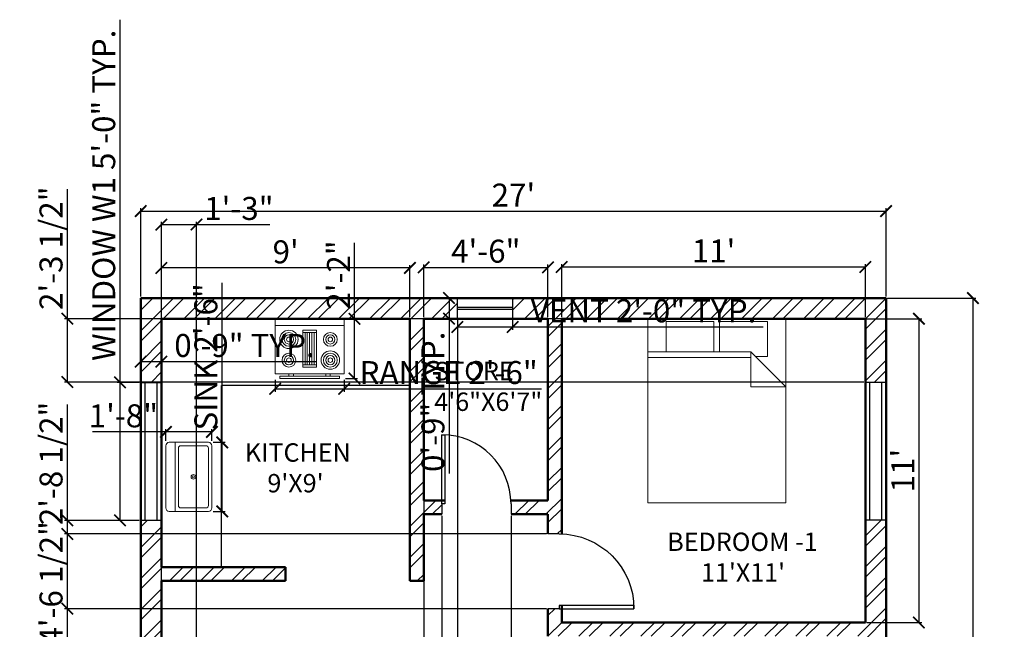
# Model space of a CAD drawing. Units: inches. Extents: x 9 to 670, y -4 to 628.
# Tile 2 of 2: x 9 to 437, y 363 to 628. Entities that reach past the tile are written whole.
import ezdxf

# ---------------------------------------------------------------- set-up
doc = ezdxf.new("R2010")
doc.units = ezdxf.units.IN
for name, color, linetype, lineweight in [('A-AREA-IDEN', 1, 'Continuous', 25), ('A-EQPM', 2, 'Continuous', 18), ('A-FLOR-CASE', 34, 'Continuous', 25), ('A-FLOR-FIXT', 2, 'Continuous', 18), ('A-FURN', 2, 'Continuous', 18), ('A-WALL-PATT', 9, 'Continuous', 13), ('DIM', 3, 'Continuous', 18), ('DOORS', 4, 'Continuous', 25), ('VENTILATOR', 11, 'Continuous', 25), ('WALLS', 6, 'Continuous', 50), ('WINDOWS', 20, 'Continuous', 25)]:
    doc.layers.add(name, color=color, linetype=linetype, lineweight=lineweight)
doc.styles.get("Standard").update_dxf_attribs({"font": 'arial.ttf'})
doc.dimstyles.new('ISO-25', dxfattribs={"dimtxt": 10, "dimasz": 5, "dimexe": 1.25, "dimexo": 0.625, "dimtad": 1, "dimlunit": 4, "dimtxsty": 'Standard', "dimblk": 'ARCHTICK', "dimcen": 2.5, "dimadec": 0, "dimazin": 0, "dimtfac": 1, "dimtmove": 0, "dimatfit": 3, "dimfxl": 1, "dimarcsym": 0})

# ---------------------------------------------------------------- blocks, each defined once
blk = doc.blocks.new('Bed - Queen')
for p, q in [((0, -80.00003), (0, 0)), ((0, 0), (59.99999, 0)), ((59.99999, 0), (59.99999, -80.00003)), ((7.99999, -1.2), (28.79998, -1.2)), ((7.99999, -14.4), (7.99999, -1.2)), ((28.79998, -1.2), (28.79998, -14.4)), ((31.19999, -1.2), (51.99999, -1.2)), ((31.19999, -14.4), (31.19999, -1.2)), ((51.99999, -1.2), (51.99999, -16.4)), ((0, -14.4), (44.8, -14.4)), ((44.8, -16.8), (0, -16.8)), ((59.99999, -29.6), (44.8, -14.4)), ((44.8, -14.4), (44.8, -29.6)), ((51.99999, -16.4), (46.79936, -16.4)), ((44.8, -29.6), (59.99999, -29.6)), ((59.99999, -80.00003), (0, -80.00003))]:
    blk.add_line(p, q)
blk = doc.blocks.new('Sink-single - 30 in top')
blk.add_line((-15, -3.999996), (15, -3.999996))
for points in [[(-13.5, 0), (13.5, 0)], [(-15, -18.499996), (-15, -1.5)], [(15, -1.5), (15, -18.499996)], [(-13.5, -17.499996), (-13.5, -6.499996)], [(-12.5, -5.499996), (12.5, -5.499996)], [(13.5, -6.499996), (13.5, -17.499996)], [(13.5, -19.999996), (-13.5, -19.999996)], [(12.5, -18.499996), (-12.5, -18.499996)]]:
    blk.add_lwpolyline(points)
for radius in [1, 0.5]:
    blk.add_circle((0, -11.999996), radius)
for centre, radius, start, end in [((-13.5, -1.5), 1.5, 90, 180), ((13.5, -1.5), 1.5, 0, 90), ((-12.5, -6.499996), 1, 90, 180), ((12.5, -6.499996), 1, 0, 90), ((-13.5, -18.499996), 1.5, 180, 270), ((-12.5, -17.499996), 1, 180, 270), ((12.5, -17.499996), 1, 270, 0), ((13.5, -18.499996), 1.5, 270, 0)]:
    blk.add_arc(centre, radius, start, end)
blk = doc.blocks.new('Range-Oven - 30 in top')
for p, q in [((0, -3), (30, -3)), ((12, -6), (18, -6)), ((13, -20), (13, -6)), ((14, -6), (14, -20)), ((15, -20), (15, -6)), ((16, -6), (16, -20)), ((17, -20), (17, -6)), ((18, -20), (12, -20)), ((6, -24), (6, -25)), ((8, -25), (8, -24)), ((22, -25), (22, -24)), ((24, -24), (24, -25))]:
    blk.add_line(p, q)
for points in [[(0, -24), (0, 0), (30, 0), (30, -24)], [(12, -21), (12, -5), (18, -5), (18, -21)], [(2, -26), (2, -25), (28, -25), (28, -26)]]:
    blk.add_lwpolyline(points, close=True)
for centre, radius in [((6, -9), 4), ((6, -9), 3), ((6, -9), 2), ((6, -9), 1), ((24, -9), 3), ((24, -9), 2), ((24, -9), 1), ((6, -18), 3), ((6, -18), 2), ((6, -18), 1), ((24, -18), 4), ((24, -18), 3), ((24, -18), 2), ((24, -18), 1)]:
    blk.add_circle(centre, radius)
blk = doc.blocks.new('*U8')
for p, q in [((0, 0), (0, -6)), ((40, 0), (40, -6))]:
    blk.add_line(p, q)
blk.add_lwpolyline([(0, 0), (0, 40), (1.75, 40), (1.75, 0)], close=True)
blk.add_arc((0, 0), 40, 0, 90)
blk = doc.blocks.new('W1')
at = {"layer": 'WINDOWS'}
for p, q in [((1078.63, 2170.04), (1087.63, 2170.04)), ((1078.63, 2110.04), (1078.63, 2170.04)), ((1080.63, 2110.04), (1080.63, 2170.04)), ((1085.63, 2170.04), (1085.63, 2110.04)), ((1087.63, 2170.04), (1087.63, 2110.04)), ((1087.63, 2110.04), (1078.63, 2110.04))]:
    blk.add_line(p, q, dxfattribs=at)
blk = doc.blocks.new('VENTILATOR')
at = {"layer": 'VENTILATOR'}
for p, q in [((1084.96, 2166.43), (1093.96, 2166.43)), ((1084.96, 2142.43), (1084.96, 2166.43)), ((1088.96, 2142.43), (1088.96, 2166.43)), ((1089.96, 2166.43), (1089.96, 2142.43)), ((1093.96, 2166.43), (1093.96, 2142.43)), ((1093.96, 2142.43), (1084.96, 2142.43))]:
    blk.add_line(p, q, dxfattribs=at)
blk = doc.blocks.new('_ArchTick')
at = {"color": 0, "linetype": 'ByBlock', "const_width": 0.15}
blk.add_lwpolyline([(-0.5, -0.5), (0.5, 0.5)], dxfattribs=at)
blk = doc.blocks.new('*D12')
at = {"layer": 'Defpoints', "color": 0, "transparency": 16777216}
for p in [(376.85, 498.12), (376.85, 366.12), (400.09, 366.12)]:
    blk.add_point(p, dxfattribs=at)
at = {"layer": 'DIM', "color": 0, "lineweight": -2, "transparency": 16777216}
for p, q in [((377.48, 498.12), (401.34, 498.12)), ((400.09, 498.12), (400.09, 366.12)), ((377.48, 366.12), (401.34, 366.12))]:
    blk.add_line(p, q, dxfattribs=at)
at = {"layer": 'DIM', "color": 0, "lineweight": -2, "transparency": 16777216, "xscale": 5, "yscale": 5, "zscale": 5}
for p, rotation in [((400.09, 498.12), 90), ((400.09, 366.12), 270)]:
    blk.add_blockref('_ArchTick', p, dxfattribs=dict(at, rotation=rotation))
at = {"layer": 'DIM', "color": 0, "transparency": 16777216, "insert": (394.44, 432.12), "char_height": 10, "attachment_point": 5, "rotation": 90}
blk.add_mtext("11'", dxfattribs=at)
blk = doc.blocks.new('*D15')
at = {"layer": 'Defpoints', "color": 0, "transparency": 16777216}
for p in [(385.85, 507.12), (385.85, 63.12), (423.57, 63.12)]:
    blk.add_point(p, dxfattribs=at)
at = {"layer": 'DIM', "color": 0, "lineweight": -2, "transparency": 16777216}
for p, q in [((386.48, 507.12), (424.82, 507.12)), ((423.57, 507.12), (423.57, 63.12)), ((386.48, 63.12), (424.82, 63.12))]:
    blk.add_line(p, q, dxfattribs=at)
at = {"layer": 'DIM', "color": 0, "lineweight": -2, "transparency": 16777216, "xscale": 5, "yscale": 5, "zscale": 5}
for p, rotation in [((423.57, 507.12), 90), ((423.57, 63.12), 270)]:
    blk.add_blockref('_ArchTick', p, dxfattribs=dict(at, rotation=rotation))
at = {"layer": 'DIM', "color": 0, "transparency": 16777216, "insert": (417.84, 285.12), "char_height": 10, "attachment_point": 5, "rotation": 90}
blk.add_mtext("37'", dxfattribs=at)
blk = doc.blocks.new('*D16')
at = {"layer": 'Defpoints', "color": 0, "transparency": 16777216}
for p in [(70.85, 520.17), (70.85, 498.12), (178.85, 498.12)]:
    blk.add_point(p, dxfattribs=at)
at = {"layer": 'DIM', "color": 0, "lineweight": -2, "transparency": 16777216}
for p, q in [((70.85, 498.74), (70.85, 521.42)), ((178.85, 520.17), (70.85, 520.17)), ((178.85, 498.74), (178.85, 521.42))]:
    blk.add_line(p, q, dxfattribs=at)
at = {"layer": 'DIM', "color": 0, "lineweight": -2, "transparency": 16777216, "xscale": 5, "yscale": 5, "zscale": 5, "rotation": 180}
blk.add_blockref('_ArchTick', (70.85, 520.17), dxfattribs=at)
at = {"layer": 'DIM', "color": 0, "lineweight": -2, "transparency": 16777216, "xscale": 5, "yscale": 5, "zscale": 5}
blk.add_blockref('_ArchTick', (178.85, 520.17), dxfattribs=at)
at = {"layer": 'DIM', "color": 0, "transparency": 16777216, "insert": (124.85, 525.9), "char_height": 10, "attachment_point": 5}
blk.add_mtext("9'", dxfattribs=at)
blk = doc.blocks.new('*D17')
at = {"layer": 'Defpoints', "color": 0, "transparency": 16777216}
for p in [(238.85, 520.44), (184.85, 498.12), (238.85, 498.12)]:
    blk.add_point(p, dxfattribs=at)
at = {"layer": 'DIM', "color": 0, "lineweight": -2, "transparency": 16777216}
for p, q in [((184.85, 498.74), (184.85, 521.69)), ((184.85, 520.44), (238.85, 520.44)), ((238.85, 498.74), (238.85, 521.69))]:
    blk.add_line(p, q, dxfattribs=at)
at = {"layer": 'DIM', "color": 0, "lineweight": -2, "transparency": 16777216, "xscale": 5, "yscale": 5, "zscale": 5, "rotation": 180}
blk.add_blockref('_ArchTick', (184.85, 520.44), dxfattribs=at)
at = {"layer": 'DIM', "color": 0, "lineweight": -2, "transparency": 16777216, "xscale": 5, "yscale": 5, "zscale": 5}
blk.add_blockref('_ArchTick', (238.85, 520.44), dxfattribs=at)
at = {"layer": 'DIM', "color": 0, "transparency": 16777216, "insert": (211.85, 526.17), "char_height": 10, "attachment_point": 5}
blk.add_mtext('4\'-6"', dxfattribs=at)
blk = doc.blocks.new('*D18')
at = {"layer": 'Defpoints', "color": 0, "transparency": 16777216}
for p in [(376.85, 520.64), (244.85, 498.12), (376.85, 498.12)]:
    blk.add_point(p, dxfattribs=at)
at = {"layer": 'DIM', "color": 0, "lineweight": -2, "transparency": 16777216}
for p, q in [((244.85, 498.74), (244.85, 521.89)), ((244.85, 520.64), (376.85, 520.64)), ((376.85, 498.74), (376.85, 521.89))]:
    blk.add_line(p, q, dxfattribs=at)
at = {"layer": 'DIM', "color": 0, "lineweight": -2, "transparency": 16777216, "xscale": 5, "yscale": 5, "zscale": 5, "rotation": 180}
blk.add_blockref('_ArchTick', (244.85, 520.64), dxfattribs=at)
at = {"layer": 'DIM', "color": 0, "lineweight": -2, "transparency": 16777216, "xscale": 5, "yscale": 5, "zscale": 5}
blk.add_blockref('_ArchTick', (376.85, 520.64), dxfattribs=at)
at = {"layer": 'DIM', "color": 0, "transparency": 16777216, "insert": (310.85, 526.28), "char_height": 10, "attachment_point": 5}
blk.add_mtext("11'", dxfattribs=at)
blk = doc.blocks.new('*D19')
at = {"layer": 'Defpoints', "color": 0, "transparency": 16777216}
for p in [(385.85, 544.91), (61.85, 507.12), (385.85, 507.12)]:
    blk.add_point(p, dxfattribs=at)
at = {"layer": 'DIM', "color": 0, "lineweight": -2, "transparency": 16777216}
for p, q in [((61.85, 507.74), (61.85, 546.16)), ((61.85, 544.91), (385.85, 544.91)), ((385.85, 507.74), (385.85, 546.16))]:
    blk.add_line(p, q, dxfattribs=at)
at = {"layer": 'DIM', "color": 0, "lineweight": -2, "transparency": 16777216, "xscale": 5, "yscale": 5, "zscale": 5, "rotation": 180}
blk.add_blockref('_ArchTick', (61.85, 544.91), dxfattribs=at)
at = {"layer": 'DIM', "color": 0, "lineweight": -2, "transparency": 16777216, "xscale": 5, "yscale": 5, "zscale": 5}
blk.add_blockref('_ArchTick', (385.85, 544.91), dxfattribs=at)
at = {"layer": 'DIM', "color": 0, "transparency": 16777216, "insert": (223.85, 550.55), "char_height": 10, "attachment_point": 5}
blk.add_mtext("27'", dxfattribs=at)
blk = doc.blocks.new('*D21')
at = {"layer": 'Defpoints', "color": 0, "transparency": 16777216}
for p in [(52.85, 470.46), (61.85, 470.46), (61.85, 410.46)]:
    blk.add_point(p, dxfattribs=at)
at = {"layer": 'DIM', "color": 0, "lineweight": -2, "transparency": 16777216}
for p, q in [((52.85, 470.46), (52.85, 628.09)), ((61.23, 470.46), (51.6, 470.46)), ((52.85, 410.46), (52.85, 470.46)), ((61.23, 410.46), (51.6, 410.46))]:
    blk.add_line(p, q, dxfattribs=at)
at = {"layer": 'DIM', "color": 0, "lineweight": -2, "transparency": 16777216, "xscale": 5, "yscale": 5, "zscale": 5}
for p, rotation in [((52.85, 470.46), 90), ((52.85, 410.46), 270)]:
    blk.add_blockref('_ArchTick', p, dxfattribs=dict(at, rotation=rotation))
at = {"layer": 'DIM', "color": 0, "transparency": 16777216, "insert": (47.05, 551.77), "char_height": 10, "attachment_point": 5, "rotation": 90}
blk.add_mtext('WINDOW W1 5\'-0" TYP.', dxfattribs=at)
blk = doc.blocks.new('*D22')
at = {"layer": 'Defpoints', "color": 0, "transparency": 16777216}
for p in [(70.85, 479.46), (61.85, 470.46), (70.85, 470.46)]:
    blk.add_point(p, dxfattribs=at)
at = {"layer": 'DIM', "color": 0, "lineweight": -2, "transparency": 16777216}
for p, q in [((61.85, 471.08), (61.85, 480.71)), ((61.85, 479.46), (70.85, 479.46)), ((70.85, 471.08), (70.85, 480.71)), ((70.85, 479.46), (138.06, 479.46))]:
    blk.add_line(p, q, dxfattribs=at)
at = {"layer": 'DIM', "color": 0, "lineweight": -2, "transparency": 16777216, "xscale": 5, "yscale": 5, "zscale": 5, "rotation": 180}
blk.add_blockref('_ArchTick', (61.85, 479.46), dxfattribs=at)
at = {"layer": 'DIM', "color": 0, "lineweight": -2, "transparency": 16777216, "xscale": 5, "yscale": 5, "zscale": 5}
blk.add_blockref('_ArchTick', (70.85, 479.46), dxfattribs=at)
at = {"layer": 'DIM', "color": 0, "transparency": 16777216, "insert": (106.95, 485.19), "char_height": 10, "attachment_point": 5}
blk.add_mtext('0\'-9" TYP.', dxfattribs=at)
blk = doc.blocks.new('*D25')
at = {"layer": 'Defpoints', "color": 0, "transparency": 16777216}
for p in [(199.5, 498.12), (223.5, 498.12), (223.5, 494.52)]:
    blk.add_point(p, dxfattribs=at)
at = {"layer": 'DIM', "color": 0, "lineweight": -2, "transparency": 16777216}
for p, q in [((199.5, 497.49), (199.5, 493.27)), ((223.5, 497.49), (223.5, 493.27)), ((199.5, 494.52), (223.5, 494.52)), ((223.5, 494.52), (332.36, 494.52))]:
    blk.add_line(p, q, dxfattribs=at)
at = {"layer": 'DIM', "color": 0, "lineweight": -2, "transparency": 16777216, "xscale": 5, "yscale": 5, "zscale": 5, "rotation": 180}
blk.add_blockref('_ArchTick', (199.5, 494.52), dxfattribs=at)
at = {"layer": 'DIM', "color": 0, "lineweight": -2, "transparency": 16777216, "xscale": 5, "yscale": 5, "zscale": 5}
blk.add_blockref('_ArchTick', (223.5, 494.52), dxfattribs=at)
at = {"layer": 'DIM', "color": 0, "transparency": 16777216, "insert": (280.43, 500.25), "char_height": 10, "attachment_point": 5}
blk.add_mtext('VENT 2\'-0" TYP.', dxfattribs=at)
blk = doc.blocks.new('*D26')
at = {"layer": 'Defpoints', "color": 0, "transparency": 16777216}
for p in [(199.5, 507.12), (195.9, 498.12), (199.5, 498.12)]:
    blk.add_point(p, dxfattribs=at)
at = {"layer": 'DIM', "color": 0, "lineweight": -2, "transparency": 16777216}
for p, q in [((198.88, 507.12), (194.65, 507.12)), ((195.9, 507.12), (195.9, 498.12)), ((198.88, 498.12), (194.65, 498.12)), ((195.9, 498.12), (195.9, 430.91))]:
    blk.add_line(p, q, dxfattribs=at)
at = {"layer": 'DIM', "color": 0, "lineweight": -2, "transparency": 16777216, "xscale": 5, "yscale": 5, "zscale": 5}
for p, rotation in [((195.9, 507.12), 90), ((195.9, 498.12), 270)]:
    blk.add_blockref('_ArchTick', p, dxfattribs=dict(at, rotation=rotation))
at = {"layer": 'DIM', "color": 0, "transparency": 16777216, "insert": (190.17, 462.02), "char_height": 10, "attachment_point": 5, "rotation": 90}
blk.add_mtext('0\'-9" TYP.', dxfattribs=at)
blk = doc.blocks.new('*D27')
at = {"layer": 'Defpoints', "color": 0, "transparency": 16777216}
for p in [(376.85, 344.96), (343.8, 340), (376.85, 340)]:
    blk.add_point(p, dxfattribs=at)
at = {"layer": 'DIM', "color": 0, "lineweight": -2, "transparency": 16777216}
for p, q in [((343.8, 340.63), (343.8, 346.21)), ((343.8, 344.96), (376.85, 344.96)), ((376.85, 340.63), (376.85, 346.21)), ((376.85, 344.96), (437.25, 344.96))]:
    blk.add_line(p, q, dxfattribs=at)
at = {"layer": 'DIM', "color": 0, "lineweight": -2, "transparency": 16777216, "xscale": 5, "yscale": 5, "zscale": 5, "rotation": 180}
blk.add_blockref('_ArchTick', (343.8, 344.96), dxfattribs=at)
at = {"layer": 'DIM', "color": 0, "lineweight": -2, "transparency": 16777216, "xscale": 5, "yscale": 5, "zscale": 5}
blk.add_blockref('_ArchTick', (376.85, 344.96), dxfattribs=at)
at = {"layer": 'DIM', "color": 0, "transparency": 16777216, "insert": (409.55, 350.75), "char_height": 10, "attachment_point": 5}
blk.add_mtext('WC 2\'-9"', dxfattribs=at)
blk = doc.blocks.new('*D31')
at = {"layer": 'Defpoints', "color": 0, "transparency": 16777216}
for p in [(92.76, 444.39), (97.26, 444.39), (92.76, 414.39)]:
    blk.add_point(p, dxfattribs=at)
at = {"layer": 'DIM', "color": 0, "lineweight": -2, "transparency": 16777216}
for p, q in [((97.26, 444.39), (97.26, 513.66)), ((93.38, 444.39), (98.51, 444.39)), ((97.26, 414.39), (97.26, 444.39)), ((93.38, 414.39), (98.51, 414.39))]:
    blk.add_line(p, q, dxfattribs=at)
at = {"layer": 'DIM', "color": 0, "lineweight": -2, "transparency": 16777216, "xscale": 5, "yscale": 5, "zscale": 5}
for p, rotation in [((97.26, 444.39), 90), ((97.26, 414.39), 270)]:
    blk.add_blockref('_ArchTick', p, dxfattribs=dict(at, rotation=rotation))
at = {"layer": 'DIM', "color": 0, "transparency": 16777216, "insert": (91.46, 481.53), "char_height": 10, "attachment_point": 5, "rotation": 90}
blk.add_mtext('SINK 2\'-6"', dxfattribs=at)
blk = doc.blocks.new('*D32')
at = {"layer": 'Defpoints', "color": 0, "transparency": 16777216}
for p in [(72.76, 448.89), (72.76, 444.39), (92.76, 444.39)]:
    blk.add_point(p, dxfattribs=at)
at = {"layer": 'DIM', "color": 0, "lineweight": -2, "transparency": 16777216}
for p, q in [((72.76, 445.02), (72.76, 450.14)), ((92.76, 445.02), (92.76, 450.14)), ((72.76, 448.89), (40.87, 448.89)), ((92.76, 448.89), (72.76, 448.89))]:
    blk.add_line(p, q, dxfattribs=at)
at = {"layer": 'DIM', "color": 0, "lineweight": -2, "transparency": 16777216, "xscale": 5, "yscale": 5, "zscale": 5, "rotation": 180}
blk.add_blockref('_ArchTick', (72.76, 448.89), dxfattribs=at)
at = {"layer": 'DIM', "color": 0, "lineweight": -2, "transparency": 16777216, "xscale": 5, "yscale": 5, "zscale": 5}
blk.add_blockref('_ArchTick', (92.76, 448.89), dxfattribs=at)
at = {"layer": 'DIM', "color": 0, "transparency": 16777216, "insert": (54.31, 454.62), "char_height": 10, "attachment_point": 5}
blk.add_mtext('1\'-8"', dxfattribs=at)
blk = doc.blocks.new('*D33')
at = {"layer": 'Defpoints', "color": 0, "transparency": 16777216}
for p in [(120.27, 472.12), (150.27, 472.12), (150.27, 467.62)]:
    blk.add_point(p, dxfattribs=at)
at = {"layer": 'DIM', "color": 0, "lineweight": -2, "transparency": 16777216}
for p, q in [((120.27, 471.49), (120.27, 466.37)), ((150.27, 471.49), (150.27, 466.37)), ((120.27, 467.62), (150.27, 467.62)), ((150.27, 467.62), (236.14, 467.62))]:
    blk.add_line(p, q, dxfattribs=at)
at = {"layer": 'DIM', "color": 0, "lineweight": -2, "transparency": 16777216, "xscale": 5, "yscale": 5, "zscale": 5, "rotation": 180}
blk.add_blockref('_ArchTick', (120.27, 467.62), dxfattribs=at)
at = {"layer": 'DIM', "color": 0, "lineweight": -2, "transparency": 16777216, "xscale": 5, "yscale": 5, "zscale": 5}
blk.add_blockref('_ArchTick', (150.27, 467.62), dxfattribs=at)
at = {"layer": 'DIM', "color": 0, "transparency": 16777216, "insert": (195.71, 473.41), "char_height": 10, "attachment_point": 5}
blk.add_mtext('RANGE 2\'-6"', dxfattribs=at)
blk = doc.blocks.new('*D34')
at = {"layer": 'Defpoints', "color": 0, "transparency": 16777216}
for p in [(150.27, 498.12), (154.77, 498.12), (150.27, 472.12)]:
    blk.add_point(p, dxfattribs=at)
at = {"layer": 'DIM', "color": 0, "lineweight": -2, "transparency": 16777216}
for p, q in [((154.77, 498.12), (154.77, 531.12)), ((150.89, 498.12), (156.02, 498.12)), ((154.77, 472.12), (154.77, 498.12)), ((150.89, 472.12), (156.02, 472.12))]:
    blk.add_line(p, q, dxfattribs=at)
at = {"layer": 'DIM', "color": 0, "lineweight": -2, "transparency": 16777216, "xscale": 5, "yscale": 5, "zscale": 5}
for p, rotation in [((154.77, 498.12), 90), ((154.77, 472.12), 270)]:
    blk.add_blockref('_ArchTick', p, dxfattribs=dict(at, rotation=rotation))
at = {"layer": 'DIM', "color": 0, "transparency": 16777216, "insert": (149.12, 517.12), "char_height": 10, "attachment_point": 5, "rotation": 90}
blk.add_mtext('2\'-2"', dxfattribs=at)
blk = doc.blocks.new('*D42')
at = {"layer": 'Defpoints', "color": 0, "transparency": 16777216}
for p in [(29.95, 404.58), (238.85, 404.58), (238.85, 372.06)]:
    blk.add_point(p, dxfattribs=at)
at = {"layer": 'DIM', "color": 0, "lineweight": -2, "transparency": 16777216}
for p, q in [((29.95, 404.58), (29.95, 460.89)), ((238.23, 404.58), (28.7, 404.58)), ((29.95, 372.06), (29.95, 404.58)), ((238.23, 372.06), (28.7, 372.06))]:
    blk.add_line(p, q, dxfattribs=at)
at = {"layer": 'DIM', "color": 0, "lineweight": -2, "transparency": 16777216, "xscale": 5, "yscale": 5, "zscale": 5}
for p, rotation in [((29.95, 404.58), 90), ((29.95, 372.06), 270)]:
    blk.add_blockref('_ArchTick', p, dxfattribs=dict(at, rotation=rotation))
at = {"layer": 'DIM', "color": 0, "transparency": 16777216, "insert": (24.16, 435.23), "char_height": 10, "attachment_point": 5, "rotation": 90}
blk.add_mtext('2\'-8 1/2"', dxfattribs=at)
blk = doc.blocks.new('*D43')
at = {"layer": 'Defpoints', "color": 0, "transparency": 16777216}
for p in [(192.78, 413.12), (222.81, 413.12), (222.81, 7.22)]:
    blk.add_point(p, dxfattribs=at)
at = {"layer": 'DIM', "color": 0, "lineweight": -2, "transparency": 16777216}
for p, q in [((192.78, 412.49), (192.78, 5.97)), ((222.81, 412.49), (222.81, 5.97)), ((192.78, 7.22), (222.81, 7.22))]:
    blk.add_line(p, q, dxfattribs=at)
at = {"layer": 'DIM', "color": 0, "lineweight": -2, "transparency": 16777216, "xscale": 5, "yscale": 5, "zscale": 5, "rotation": 180}
blk.add_blockref('_ArchTick', (192.78, 7.22), dxfattribs=at)
at = {"layer": 'DIM', "color": 0, "lineweight": -2, "transparency": 16777216, "xscale": 5, "yscale": 5, "zscale": 5}
blk.add_blockref('_ArchTick', (222.81, 7.22), dxfattribs=at)
at = {"layer": 'DIM', "color": 0, "transparency": 16777216, "insert": (207.8, 12.95), "char_height": 10, "attachment_point": 5}
blk.add_mtext('2\'-6"', dxfattribs=at)
blk = doc.blocks.new('*D46')
at = {"layer": 'Defpoints', "color": 0, "transparency": 16777216}
for p in [(29.95, 410.46), (61.85, 410.46), (61.85, 356.16)]:
    blk.add_point(p, dxfattribs=at)
at = {"layer": 'DIM', "color": 0, "lineweight": -2, "transparency": 16777216}
for p, q in [((61.23, 410.46), (28.7, 410.46)), ((29.95, 356.16), (29.95, 410.46)), ((61.23, 356.16), (28.7, 356.16))]:
    blk.add_line(p, q, dxfattribs=at)
at = {"layer": 'DIM', "color": 0, "lineweight": -2, "transparency": 16777216, "xscale": 5, "yscale": 5, "zscale": 5}
for p, rotation in [((29.95, 410.46), 90), ((29.95, 356.16), 270)]:
    blk.add_blockref('_ArchTick', p, dxfattribs=dict(at, rotation=rotation))
at = {"layer": 'DIM', "color": 0, "transparency": 16777216, "insert": (24.16, 383.31), "char_height": 10, "attachment_point": 5, "rotation": 90}
blk.add_mtext('4\'-6 1/2"', dxfattribs=at)
blk = doc.blocks.new('*D47')
at = {"layer": 'Defpoints', "color": 0, "transparency": 16777216}
for p in [(86.08, 539.02), (70.85, 72.12), (86.08, 72.12)]:
    blk.add_point(p, dxfattribs=at)
at = {"layer": 'DIM', "color": 0, "lineweight": -2, "transparency": 16777216}
for p, q in [((70.85, 72.74), (70.85, 540.27)), ((86.08, 72.74), (86.08, 540.27)), ((70.85, 539.02), (86.08, 539.02)), ((86.08, 539.02), (117.98, 539.02))]:
    blk.add_line(p, q, dxfattribs=at)
at = {"layer": 'DIM', "color": 0, "lineweight": -2, "transparency": 16777216, "xscale": 5, "yscale": 5, "zscale": 5, "rotation": 180}
blk.add_blockref('_ArchTick', (70.85, 539.02), dxfattribs=at)
at = {"layer": 'DIM', "color": 0, "lineweight": -2, "transparency": 16777216, "xscale": 5, "yscale": 5, "zscale": 5}
blk.add_blockref('_ArchTick', (86.08, 539.02), dxfattribs=at)
at = {"layer": 'DIM', "color": 0, "transparency": 16777216, "insert": (104.53, 544.75), "char_height": 10, "attachment_point": 5}
blk.add_mtext('1\'-3"', dxfattribs=at)
blk = doc.blocks.new('*D48')
at = {"layer": 'Defpoints', "color": 0, "transparency": 16777216}
for p in [(184.85, 498.12), (199.5, 498.12), (199.5, 7.22)]:
    blk.add_point(p, dxfattribs=at)
at = {"layer": 'DIM', "color": 0, "lineweight": -2, "transparency": 16777216}
for p, q in [((184.85, 497.49), (184.85, 5.97)), ((199.5, 497.49), (199.5, 5.97)), ((184.85, 7.22), (199.5, 7.22)), ((199.5, 7.22), (254.69, 7.22))]:
    blk.add_line(p, q, dxfattribs=at)
at = {"layer": 'DIM', "color": 0, "lineweight": -2, "transparency": 16777216, "xscale": 5, "yscale": 5, "zscale": 5, "rotation": 180}
blk.add_blockref('_ArchTick', (184.85, 7.22), dxfattribs=at)
at = {"layer": 'DIM', "color": 0, "lineweight": -2, "transparency": 16777216, "xscale": 5, "yscale": 5, "zscale": 5}
blk.add_blockref('_ArchTick', (199.5, 7.22), dxfattribs=at)
at = {"layer": 'DIM', "color": 0, "transparency": 16777216, "insert": (229.6, 13.01), "char_height": 10, "attachment_point": 5}
blk.add_mtext('1\'-2 1/2"', dxfattribs=at)
blk = doc.blocks.new('*D49')
at = {"layer": 'Defpoints', "color": 0, "transparency": 16777216}
for p in [(29.95, 498.12), (376.85, 498.12), (376.85, 470.6)]:
    blk.add_point(p, dxfattribs=at)
at = {"layer": 'DIM', "color": 0, "lineweight": -2, "transparency": 16777216}
for p, q in [((29.95, 498.12), (29.95, 554.42)), ((376.23, 498.12), (28.7, 498.12)), ((29.95, 470.6), (29.95, 498.12)), ((376.23, 470.6), (28.7, 470.6))]:
    blk.add_line(p, q, dxfattribs=at)
at = {"layer": 'DIM', "color": 0, "lineweight": -2, "transparency": 16777216, "xscale": 5, "yscale": 5, "zscale": 5}
for p, rotation in [((29.95, 498.12), 90), ((29.95, 470.6), 270)]:
    blk.add_blockref('_ArchTick', p, dxfattribs=dict(at, rotation=rotation))
at = {"layer": 'DIM', "color": 0, "transparency": 16777216, "insert": (24.15, 528.77), "char_height": 10, "attachment_point": 5, "rotation": 90}
blk.add_mtext('2\'-3 1/2"', dxfattribs=at)

msp = doc.modelspace()

# ---------------------------------------------------------------- hatches: boundary and pattern name
at = {"layer": 'A-WALL-PATT'}
h = msp.add_hatch(dxfattribs=at)
h.set_pattern_fill('ANSI32', color=256)
h.paths.add_polyline_path([(70.851, 384.119), (124.851, 384.119), (124.851, 390.119), (70.851, 390.119), (70.851, 410.46), (61.851, 410.46), (61.851, 356.162), (70.851, 356.162)])
h.paths.add_polyline_path([(199.501, 507.119), (61.851, 507.119), (61.851, 470.46), (70.851, 470.46), (70.851, 498.119), (178.851, 498.119), (178.851, 384.119), (184.851, 384.119), (184.851, 413.119), (192.784, 413.119), (192.784, 417.623), (192.784, 419.119), (184.851, 419.119), (184.851, 498.119), (199.501, 498.119)])
h.paths.add_polyline_path([(244.851, 498.119), (376.851, 498.119), (376.851, 470.602), (385.851, 470.602), (385.851, 507.119), (223.501, 507.119), (223.501, 498.119), (238.851, 498.119), (238.851, 419.119), (222.776, 419.119, -0.0124579), (222.813, 417.623), (222.813, 413.119), (238.851, 413.119), (238.851, 404.582), (243.729, 404.582, -0.0086282), (244.851, 404.563)])
h.paths.add_polyline_path([(385.851, 410.602), (376.851, 410.602), (376.851, 366.119), (244.851, 366.119), (244.851, 372.063), (243.729, 372.063), (238.851, 372.063), (238.851, 360.119), (286.851, 360.119), (286.851, 351.292), (291.355, 351.292), (292.851, 351.292), (292.851, 360.119), (376.851, 360.119), (376.851, 340), (385.851, 340)])
h.paths.add_polyline_path([(385.851, 188.838), (376.851, 188.838), (376.851, 149.119), (244.851, 149.119), (244.851, 288.119), (249.83, 288.119), (249.83, 289.241), (249.83, 294.119), (238.851, 294.119), (238.851, 246.119), (220.031, 246.119), (220.031, 244.997), (220.031, 240.119), (238.851, 240.119), (238.851, 143.119), (244.851, 143.119), (376.851, 143.119), (376.851, 130.511), (385.851, 130.511)])
h.paths.add_polyline_path([(385.851, 316), (376.851, 316), (376.851, 294.119), (292.851, 294.119), (292.851, 321.301, -0.0124579), (291.355, 321.264), (286.851, 321.264), (286.851, 294.119), (282.349, 294.119), (282.349, 289.241, -0.0086282), (282.33, 288.119), (376.851, 288.119), (376.851, 248.838), (385.851, 248.838)])
h.paths.add_polyline_path([(187.53, 246.119), (70.851, 246.119), (70.851, 296.162), (61.851, 296.162), (61.851, 190.214), (70.851, 190.214), (70.851, 240.119), (187.511, 240.119), (187.511, 244.997, -0.0086282)])
h.paths.add_polyline_path([(385.851, 82.511), (376.851, 82.511), (376.851, 72.119), (221.899, 72.119, -0.0187698), (222.012, 69.119), (222.012, 63.119), (385.851, 63.119)])
h.paths.add_polyline_path([(182.012, 69.119), (182.012, 72.119), (146.085, 72.119), (146.085, 63.119), (182.012, 63.119)])
h.paths.add_polyline_path([(86.085, 72.119), (70.851, 72.119), (70.851, 130.214), (61.851, 130.214), (61.851, 63.119), (86.085, 63.119)])

# ---------------------------------------------------------------- linework, layer by layer
at = {"layer": 'A-FLOR-CASE'}
for p in [(178.851, 469.13), (97.001, 390.119)]:
    msp.add_line(p, (97.001, 469.13), dxfattribs=at)
at = {"layer": 'WALLS'}
for p, q in [((61.851, 507.119), (385.851, 507.119)), ((61.851, 507.119), (61.851, 63.119)), ((385.851, 507.119), (385.851, 63.119)), ((70.851, 498.119), (178.851, 498.119)), ((70.851, 498.119), (70.851, 390.119)), ((178.851, 498.119), (178.851, 384.119)), ((184.851, 498.119), (184.851, 419.119)), ((184.851, 498.119), (238.851, 498.119)), ((238.851, 498.119), (238.851, 419.119)), ((244.851, 498.119), (244.851, 404.563)), ((244.851, 498.119), (376.851, 498.119)), ((376.851, 498.119), (376.851, 366.119)), ((184.851, 419.119), (194.098, 419.119)), ((222.776, 419.119), (238.851, 419.119)), ((184.851, 413.119), (192.784, 413.119)), ((184.851, 413.119), (184.851, 384.119)), ((222.813, 413.119), (238.851, 413.119)), ((238.851, 413.119), (238.851, 404.582)), ((70.851, 390.119), (124.851, 390.119)), ((124.851, 390.119), (124.851, 384.119)), ((70.851, 384.119), (124.851, 384.119)), ((70.851, 384.119), (70.851, 246.119)), ((178.851, 384.119), (184.851, 384.119)), ((244.851, 373.486), (244.851, 366.119)), ((238.851, 372.063), (238.851, 360.119)), ((244.851, 366.119), (376.851, 366.119))]:
    msp.add_line(p, q, dxfattribs=at)

# ---------------------------------------------------------------- block references
at = {"layer": 'A-EQPM'}
msp.add_blockref('Range-Oven - 30 in top', (120.269, 498.119), dxfattribs=at)
at = {"layer": 'A-FLOR-FIXT', "rotation": 90}
msp.add_blockref('Sink-single - 30 in top', (72.76, 429.39), dxfattribs=at)
at = {"layer": 'A-FURN'}
msp.add_blockref('Bed - Queen', (282.244, 498.119), dxfattribs=at)
at = {"layer": 'DOORS', "xscale": 0.750718739775508, "yscale": 0.750718739775508, "zscale": 0.750718739775508}
msp.add_blockref('*U8', (192.784, 417.623), dxfattribs=at)
at = {"layer": 'DOORS', "xscale": -0.812986333406137, "yscale": 0.812986333406137, "zscale": 0.812986333406137, "rotation": 270}
msp.add_blockref('*U8', (243.729, 372.063), dxfattribs=at)
at = {"layer": 'VENTILATOR', "rotation": 270}
msp.add_blockref('VENTILATOR', (-1942.925, 1592.08), dxfattribs=at)
at = {"layer": 'WINDOWS'}
for p in [(-1016.781, -1699.584), (-701.781, -1699.443)]:
    msp.add_blockref('W1', p, dxfattribs=at)

# ---------------------------------------------------------------- texts
at = {"layer": 'A-AREA-IDEN', "char_height": 8, "attachment_point": 1}
for s, width, insert in [('  STORE    \\P  4\'6"X6\'7"', 58.62227, (184.591, 479.379)), ("KITCHEN     \\P    9'X9'", 58.62227, (107.133, 443.964)), ("BEDROOM -1    \\P      11'X11'", 76.76666, (290.74, 405.168))]:
    msp.add_mtext_dynamic_manual_height_columns(s, width=width, gutter_width=12.5, heights=[0], dxfattribs=dict(at, insert=insert))

# ---------------------------------------------------------------- dimensions: what is measured, and where the dimension line sits
at = {"layer": 'DIM'}
for base, p1, p2, angle, text, picture, middle in [((52.851, 470.46), (61.851, 410.46), (61.851, 470.46), 90, 'WINDOW W1 <> TYP.', '*D21', (47.052, 551.774)), ((97.26, 444.39), (92.76, 414.39), (92.76, 444.39), 90, 'SINK <>', '*D31', (91.464, 481.526)), ((195.901, 498.119), (199.501, 507.119), (199.501, 498.119), 270, '<> TYP.', '*D26', (190.17, 462.016))]:
    dim = msp.add_linear_dim(base=base, p1=p1, p2=p2, angle=angle, text=text, dimstyle='ISO-25', override={"dimdec": 1, "dimlfac": 1, "dimrnd": 0, "dimzin": 1, "dimdsep": 46, "dimlunit": 4, "dimfrac": 2}, dxfattribs=at)
    dim.commit()
    dim.dimension.update_dxf_attribs({"geometry": picture, "text_midpoint": middle})
for base, p1, p2, override, picture, middle in [((385.851, 544.909), (61.851, 507.119), (385.851, 507.119), {"dimclrd": 0, "dimclre": 0, "dimclrt": 0}, '*D19', (223.851, 550.554)), ((86.085, 539.019), (70.851, 72.119), (86.085, 72.119), {"dimdec": 1, "dimlfac": 1, "dimrnd": 0, "dimzin": 1, "dimdsep": 46, "dimlunit": 4, "dimfrac": 2}, '*D47', (104.53, 544.753)), ((70.851, 520.174), (178.851, 498.119), (70.851, 498.119), {"dimclrd": 0, "dimclre": 0, "dimclrt": 0}, '*D16', (124.851, 525.905)), ((238.851, 520.441), (184.851, 498.119), (238.851, 498.119), {"dimclrd": 0, "dimclre": 0, "dimclrt": 0}, '*D17', (211.851, 526.171)), ((376.851, 520.636), (244.851, 498.119), (376.851, 498.119), {"dimclrd": 0, "dimclre": 0, "dimclrt": 0}, '*D18', (310.851, 526.281)), ((199.5011, 7.2188), (184.8509, 498.1188), (199.5011, 498.1188), {"dimdec": 1, "dimlfac": 1, "dimrnd": 0, "dimzin": 1, "dimdsep": 46, "dimlunit": 4, "dimfrac": 2}, '*D48', (229.5975, 13.0143)), ((222.813, 7.219), (192.784, 413.119), (222.813, 413.119), {"dimdec": 1, "dimlfac": 1, "dimrnd": 0, "dimzin": 1, "dimdsep": 46, "dimlunit": 4, "dimfrac": 2}, '*D43', (207.799, 12.95))]:
    dim = msp.add_linear_dim(base=base, p1=p1, p2=p2, dimstyle='ISO-25', override=override, dxfattribs=at)
    dim.commit()
    dim.dimension.update_dxf_attribs({"geometry": picture, "text_midpoint": middle})
for base, p1, p2, angle, override, picture, middle in [((29.951, 498.119), (376.851, 470.602), (376.851, 498.119), 90, {"dimdec": 1, "dimlfac": 1, "dimrnd": 0, "dimzin": 1, "dimdsep": 46, "dimlunit": 4, "dimfrac": 2}, '*D49', (24.152, 528.771)), ((154.769, 498.119), (150.269, 472.119), (150.269, 498.119), 90, {"dimdec": 1, "dimlfac": 1, "dimrnd": 0, "dimzin": 1, "dimdsep": 46, "dimlunit": 4, "dimfrac": 2}, '*D34', (149.123, 517.12)), ((423.574, 63.119), (385.851, 507.119), (385.851, 63.119), 90, {"dimclrd": 0, "dimclre": 0, "dimclrt": 0}, '*D15', (417.839, 285.119)), ((400.087, 366.119), (376.851, 498.119), (376.851, 366.119), 90, {"dimclrd": 0, "dimclre": 0, "dimclrt": 0}, '*D12', (394.441, 432.119)), ((29.951, 404.582), (238.851, 372.063), (238.851, 404.582), 90, {"dimdec": 1, "dimlfac": 1, "dimrnd": 0, "dimzin": 1, "dimdsep": 46, "dimlunit": 4, "dimfrac": 2}, '*D42', (24.155, 435.235)), ((72.76, 448.89), (92.76, 444.39), (72.76, 444.39), 180, {"dimdec": 1, "dimlfac": 1, "dimrnd": 0, "dimzin": 1, "dimdsep": 46, "dimlunit": 4, "dimfrac": 2}, '*D32', (54.314, 454.621)), ((29.951, 410.46), (61.851, 356.162), (61.851, 410.46), 90, {"dimdec": 1, "dimlfac": 1, "dimrnd": 0, "dimzin": 1, "dimdsep": 46, "dimlunit": 4, "dimfrac": 2}, '*D46', (24.155, 383.311))]:
    dim = msp.add_linear_dim(base=base, p1=p1, p2=p2, angle=angle, dimstyle='ISO-25', override=override, dxfattribs=at)
    dim.commit()
    dim.dimension.update_dxf_attribs({"geometry": picture, "text_midpoint": middle})
for base, p1, p2, text, picture, middle in [((223.501, 494.519), (199.501, 498.119), (223.501, 498.119), 'VENT <> TYP.', '*D25', (280.432, 500.25)), ((70.851, 479.46), (61.851, 470.46), (70.851, 470.46), '<> TYP.', '*D22', (106.953, 485.191)), ((150.269, 467.619), (120.269, 472.119), (150.269, 472.119), 'RANGE <>', '*D33', (195.706, 473.414)), ((376.851, 344.957), (343.805, 340), (376.851, 340), 'WC <>', '*D27', (409.55, 350.753))]:
    dim = msp.add_linear_dim(base=base, p1=p1, p2=p2, text=text, dimstyle='ISO-25', override={"dimdec": 1, "dimlfac": 1, "dimrnd": 0, "dimzin": 1, "dimdsep": 46, "dimlunit": 4, "dimfrac": 2}, dxfattribs=at)
    dim.commit()
    dim.dimension.update_dxf_attribs({"geometry": picture, "text_midpoint": middle})

doc.saveas('drawing.dxf')
